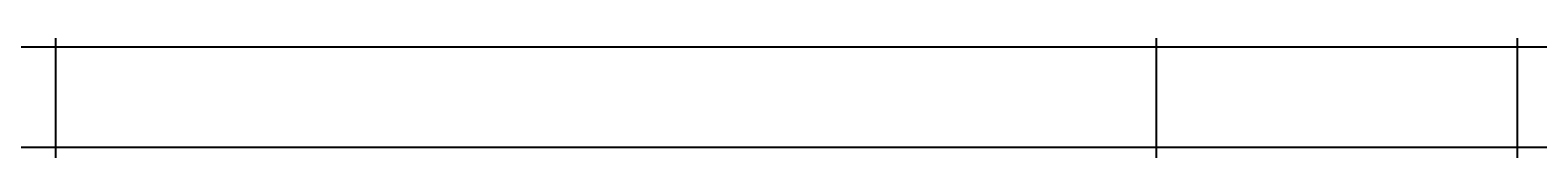
# Model space of a CAD drawing. Units: inches. Extents: x 35362 to 73946, y 43607 to 67532.
# Tile 82 of 134: x 50119 to 51337, y 47543 to 47625. Entities that reach past the tile are written whole.
import ezdxf

# ---------------------------------------------------------------- set-up
doc = ezdxf.new("R2010")
doc.units = ezdxf.units.IN
doc.header["$MEASUREMENT"] = 0
doc.layers.add('A-ANNO-DIMS', color=2, linetype='Continuous', lineweight=18)
doc.styles.get("Standard").update_dxf_attribs({"font": 'arial.ttf'})
doc.dimstyles.get("Standard").update_dxf_attribs({"dimtxt": 0.18, "dimasz": 0.18, "dimexe": 0.18, "dimexo": 0.0625, "dimgap": 0.09, "dimtad": 0, "dimtih": 1, "dimtoh": 1, "dimdec": 4, "dimzin": 0, "dimdsep": 46, "dimtxsty": 'Standard', "dimcen": 0.09, "dimadec": 0, "dimazin": 0, "dimtfac": 1, "dimtdec": 4, "dimtofl": 0, "dimtmove": 0, "dimatfit": 3, "dimfxl": 1, "dimtolj": 1, "dimtzin": 0, "dimarcsym": 0})

# ---------------------------------------------------------------- blocks, each defined once
blk = doc.blocks.new('*D11')
at = {"layer": 'A-ANNO-DIMS', "color": 0, "lineweight": -2, "transparency": 16777216}
for p, q in [((47978.7, 56028.8), (47978.7, 43606.7)), ((53109.8, 56028.8), (53109.8, 43606.7)), ((47978.8, 43606.9), (50543.9, 43606.9)), ((53109.6, 43606.9), (50544.6, 43606.9))]:
    blk.add_line(p, q, dxfattribs=at)
at = {"layer": 'A-ANNO-DIMS', "color": 0, "transparency": 16777216}
for points in [[(47978.8, 43606.9), (47978.8, 43606.8), (47978.7, 43606.9)], [(53109.6, 43606.9), (53109.6, 43606.8), (53109.8, 43606.9)]]:
    blk.add_solid(points, dxfattribs=at)
at = {"layer": 'Defpoints', "color": 0, "transparency": 16777216}
for p in [(47978.7, 56028.8), (53109.8, 56028.8), (53109.8, 43606.9)]:
    blk.add_point(p, dxfattribs=at)
at = {"layer": 'A-ANNO-DIMS', "color": 0, "transparency": 16777216, "insert": (50544.2, 43606.9), "char_height": 0.18, "attachment_point": 5}
blk.add_mtext('\\A1;5131', dxfattribs=at)
blk = doc.blocks.new('*D13')
at = {"layer": 'A-ANNO-DIMS', "color": 0, "lineweight": -2, "transparency": 16777216}
for p, q in [((48373.5, 51694), (48373.5, 43606.7)), ((51029, 51694), (51029, 43606.7)), ((48373.7, 43606.9), (49700.8, 43606.9)), ((51028.9, 43606.9), (49701.7, 43606.9))]:
    blk.add_line(p, q, dxfattribs=at)
at = {"layer": 'A-ANNO-DIMS', "color": 0, "transparency": 16777216}
for points in [[(48373.7, 43606.9), (48373.7, 43606.8), (48373.5, 43606.9)], [(51028.9, 43606.9), (51028.9, 43606.8), (51029, 43606.9)]]:
    blk.add_solid(points, dxfattribs=at)
at = {"layer": 'Defpoints', "color": 0, "transparency": 16777216}
for p in [(48373.5, 51694.1), (51029, 51694.1), (51029, 43606.9)]:
    blk.add_point(p, dxfattribs=at)
at = {"layer": 'A-ANNO-DIMS', "color": 0, "transparency": 16777216, "insert": (49701.3, 43606.9), "char_height": 0.18, "attachment_point": 5}
blk.add_mtext('\\A1;2655.6', dxfattribs=at)
blk = doc.blocks.new('*D17')
at = {"layer": 'A-ANNO-DIMS', "color": 0, "lineweight": -2, "transparency": 16777216}
for p, q in [((49923.3, 61293.2), (49923.3, 43606.7)), ((51913.9, 61293.2), (51913.9, 43606.7)), ((49923.5, 43606.9), (50918.2, 43606.9)), ((51913.8, 43606.9), (50919.1, 43606.9))]:
    blk.add_line(p, q, dxfattribs=at)
at = {"layer": 'A-ANNO-DIMS', "color": 0, "transparency": 16777216}
for points in [[(49923.5, 43606.9), (49923.5, 43606.8), (49923.3, 43606.9)], [(51913.8, 43606.9), (51913.8, 43606.8), (51913.9, 43606.9)]]:
    blk.add_solid(points, dxfattribs=at)
at = {"layer": 'Defpoints', "color": 0, "transparency": 16777216}
for p in [(49923.3, 61293.3), (51913.9, 61293.3), (51913.9, 43606.9)]:
    blk.add_point(p, dxfattribs=at)
at = {"layer": 'A-ANNO-DIMS', "color": 0, "transparency": 16777216, "insert": (50918.6, 43606.9), "char_height": 0.18, "attachment_point": 5}
blk.add_mtext('\\A1;1990.6', dxfattribs=at)
blk = doc.blocks.new('*D43')
at = {"layer": 'A-ANNO-DIMS', "color": 0, "lineweight": -2, "transparency": 16777216}
for p, q in [((62004.7, 47625.2), (35361.8, 47625.2)), ((35361.9, 47625), (35361.9, 47416.9)), ((35361.9, 47208.4), (35361.9, 47416.5)), ((62004.7, 47208.2), (35361.8, 47208.2))]:
    blk.add_line(p, q, dxfattribs=at)
at = {"layer": 'A-ANNO-DIMS', "color": 0, "transparency": 16777216}
for points in [[(35361.9, 47625), (35362, 47625), (35361.9, 47625.2)], [(35361.9, 47208.4), (35362, 47208.4), (35361.9, 47208.2)]]:
    blk.add_solid(points, dxfattribs=at)
at = {"layer": 'Defpoints', "color": 0, "transparency": 16777216}
for p in [(62004.7, 47625.2), (35361.9, 47208.2), (62004.7, 47208.2)]:
    blk.add_point(p, dxfattribs=at)
at = {"layer": 'A-ANNO-DIMS', "color": 0, "transparency": 16777216, "insert": (35361.9, 47416.7), "char_height": 0.18, "attachment_point": 5}
blk.add_mtext('\\A1;416.9', dxfattribs=at)
blk = doc.blocks.new('*D67')
at = {"layer": 'A-ANNO-DIMS', "color": 0, "lineweight": -2, "transparency": 16777216}
for p, q in [((56873.5, 53351.5), (35361.8, 53351.5)), ((35361.9, 53351.3), (35361.9, 49400.9)), ((35361.9, 45450.1), (35361.9, 49400.5)), ((53793.6, 45449.9), (35361.8, 45449.9))]:
    blk.add_line(p, q, dxfattribs=at)
at = {"layer": 'A-ANNO-DIMS', "color": 0, "transparency": 16777216}
for points in [[(35361.9, 53351.3), (35362, 53351.3), (35361.9, 53351.5)], [(35361.9, 45450.1), (35362, 45450.1), (35361.9, 45449.9)]]:
    blk.add_solid(points, dxfattribs=at)
at = {"layer": 'Defpoints', "color": 0, "transparency": 16777216}
for p in [(35361.9, 53351.5), (56873.6, 53351.5), (53793.6, 45449.9)]:
    blk.add_point(p, dxfattribs=at)
at = {"layer": 'A-ANNO-DIMS', "color": 0, "transparency": 16777216, "insert": (35361.9, 49400.7), "char_height": 0.18, "attachment_point": 5}
blk.add_mtext('\\A1;7901.6', dxfattribs=at)
blk = doc.blocks.new('*D87')
at = {"layer": 'A-ANNO-DIMS', "color": 0, "lineweight": -2, "transparency": 16777216}
for p, q in [((52362.5, 48318.3), (35361.8, 48318.3)), ((35361.9, 48318.1), (35361.9, 47931.4)), ((35361.9, 47544.3), (35361.9, 47931)), ((52362.5, 47544.1), (35361.8, 47544.1))]:
    blk.add_line(p, q, dxfattribs=at)
at = {"layer": 'A-ANNO-DIMS', "color": 0, "transparency": 16777216}
for points in [[(35361.9, 48318.1), (35362, 48318.1), (35361.9, 48318.3)], [(35361.9, 47544.3), (35362, 47544.3), (35361.9, 47544.1)]]:
    blk.add_solid(points, dxfattribs=at)
at = {"layer": 'Defpoints', "color": 0, "transparency": 16777216}
for p in [(35361.9, 48318.3), (52362.6, 48318.3), (52362.6, 47544.1)]:
    blk.add_point(p, dxfattribs=at)
at = {"layer": 'A-ANNO-DIMS', "color": 0, "transparency": 16777216, "insert": (35361.9, 47931.2), "char_height": 0.18, "attachment_point": 5}
blk.add_mtext('\\A1;774.1', dxfattribs=at)
blk = doc.blocks.new('*D107')
at = {"layer": 'A-ANNO-DIMS', "color": 0, "lineweight": -2, "transparency": 16777216}
for p, q in [((50139.6, 59850), (50139.6, 43606.7)), ((51320.8, 59850), (51320.8, 43606.7)), ((50139.7, 43606.9), (50729.7, 43606.9)), ((51320.6, 43606.9), (50730.6, 43606.9))]:
    blk.add_line(p, q, dxfattribs=at)
at = {"layer": 'A-ANNO-DIMS', "color": 0, "transparency": 16777216}
for points in [[(50139.7, 43606.9), (50139.7, 43606.8), (50139.6, 43606.9)], [(51320.6, 43606.9), (51320.6, 43606.8), (51320.8, 43606.9)]]:
    blk.add_solid(points, dxfattribs=at)
at = {"layer": 'Defpoints', "color": 0, "transparency": 16777216}
for p in [(50139.6, 59850.1), (51320.8, 59850.1), (51320.8, 43606.9)]:
    blk.add_point(p, dxfattribs=at)
at = {"layer": 'A-ANNO-DIMS', "color": 0, "transparency": 16777216, "insert": (50730.2, 43606.9), "char_height": 0.18, "attachment_point": 5}
blk.add_mtext('\\A1;1181.3', dxfattribs=at)

msp = doc.modelspace()

# ---------------------------------------------------------------- dimensions: what is measured, and where the dimension line sits
at = {"layer": 'A-ANNO-DIMS'}
for base, p1, p2, override, picture, middle in [((51913.931, 43606.859), (49923.307, 61293.286), (51913.931, 61293.286), {"dimdec": 1, "dimlfac": 1, "dimrnd": 0, "dimzin": 0, "dimdsep": 46, "dimlunit": 2}, '*D17', (50918.619, 43606.859)), ((51320.8133, 43606.859), (50139.5627, 59850.0769), (51320.8133, 59850.0769), {"dimdec": 1, "dimlfac": 1, "dimrnd": 0, "dimzin": 0, "dimdsep": 46, "dimlunit": 2}, '*D107', (50730.188, 43606.859)), ((53109.76, 43606.859), (47978.665, 56028.836), (53109.76, 56028.836), {"dimdec": 0, "dimlfac": 1, "dimrnd": 0, "dimzin": 0, "dimdsep": 46, "dimlunit": 2}, '*D11', (50544.212, 43606.859)), ((51029.043, 43606.859), (48373.492, 51694.087), (51029.043, 51694.087), {"dimdec": 1, "dimlfac": 1, "dimrnd": 0, "dimzin": 0, "dimdsep": 46, "dimlunit": 2}, '*D13', (49701.267, 43606.859))]:
    dim = msp.add_linear_dim(base=base, p1=p1, p2=p2, dimstyle='Standard', override=override, dxfattribs=at)
    dim.commit()
    dim.dimension.update_dxf_attribs({"geometry": picture, "text_midpoint": middle})
for base, p1, p2, picture, middle in [((35361.949, 53351.529), (53793.638, 45449.894), (56873.602, 53351.529), '*D67', (35361.949, 49400.712)), ((35361.949, 48318.269), (52362.557, 47544.134), (52362.557, 48318.269), '*D87', (35361.949, 47931.201)), ((35361.949, 47208.25), (62004.728, 47625.181), (62004.728, 47208.25), '*D43', (35361.949, 47416.715))]:
    dim = msp.add_linear_dim(base=base, p1=p1, p2=p2, angle=90, dimstyle='Standard', override={"dimdec": 1, "dimlfac": 1, "dimrnd": 0, "dimzin": 0, "dimdsep": 46, "dimlunit": 2}, dxfattribs=at)
    dim.commit()
    dim.dimension.update_dxf_attribs({"geometry": picture, "text_midpoint": middle})

doc.saveas('drawing.dxf')
